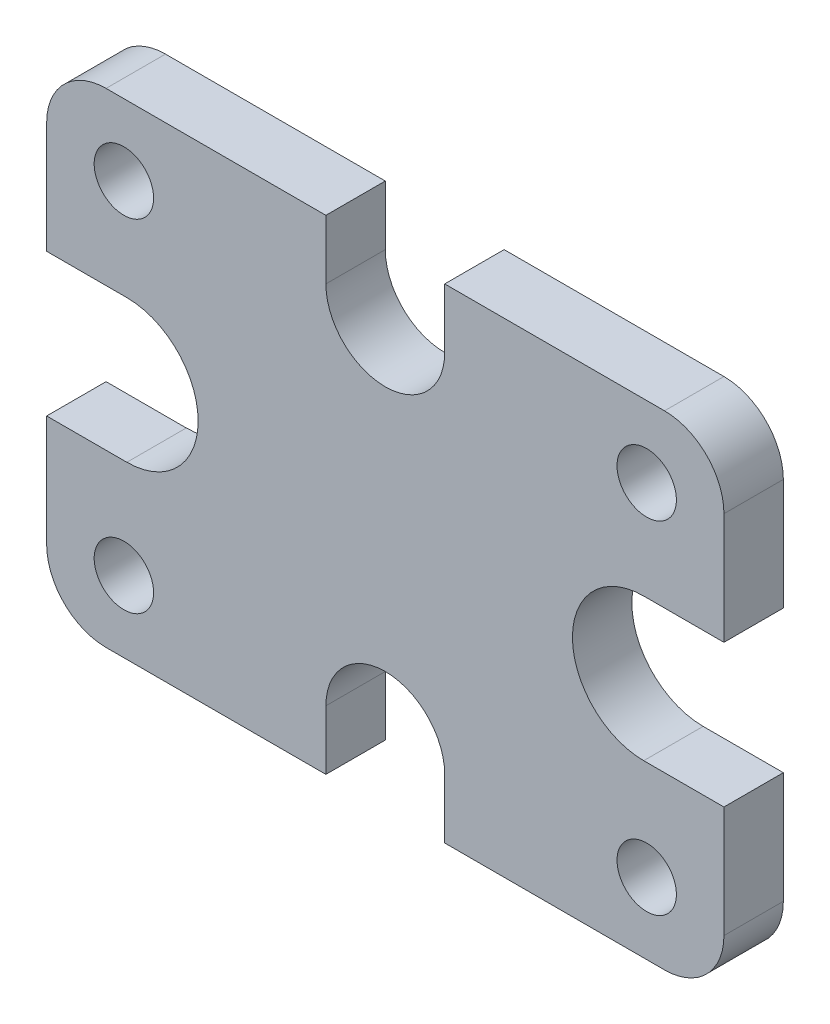
ISO-10303-21;
HEADER;
FILE_DESCRIPTION(('STEP AP214'),'2;1');
FILE_NAME('part.step','',(''),(''),'','','');
FILE_SCHEMA(('AUTOMOTIVE_DESIGN { 1 0 10303 214 1 1 1 1 }'));
ENDSEC;
DATA;
#1=APPLICATION_CONTEXT('core data for automotive mechanical design processes');
#2=APPLICATION_PROTOCOL_DEFINITION('international standard','automotive_design',2000,#1);
#3=PRODUCT_CONTEXT('',#1,'mechanical');
#4=PRODUCT('Part','Part','',(#3));
#5=PRODUCT_RELATED_PRODUCT_CATEGORY('part','',(#4));
#6=PRODUCT_DEFINITION_FORMATION('','',#4);
#7=PRODUCT_DEFINITION_CONTEXT('part definition',#1,'design');
#8=PRODUCT_DEFINITION('design','',#6,#7);
#9=PRODUCT_DEFINITION_SHAPE('','',#8);
#10=(LENGTH_UNIT() NAMED_UNIT(*) SI_UNIT(.MILLI.,.METRE.));
#11=(NAMED_UNIT(*) PLANE_ANGLE_UNIT() SI_UNIT($,.RADIAN.));
#12=(NAMED_UNIT(*) SI_UNIT($,.STERADIAN.) SOLID_ANGLE_UNIT());
#13=UNCERTAINTY_MEASURE_WITH_UNIT(LENGTH_MEASURE(1.E-05),#10,'distance_accuracy_value','');
#14=(GEOMETRIC_REPRESENTATION_CONTEXT(3) GLOBAL_UNCERTAINTY_ASSIGNED_CONTEXT((#13)) GLOBAL_UNIT_ASSIGNED_CONTEXT((#10,
#11,#12)) REPRESENTATION_CONTEXT('',''));
#15=CARTESIAN_POINT('',(0.,0.,0.));
#16=DIRECTION('',(0.,0.,1.));
#17=DIRECTION('',(1.,0.,0.));
#18=AXIS2_PLACEMENT_3D('',#15,#16,#17);
#19=CARTESIAN_POINT('',(10.0000000000001,0.,10.));
#20=DIRECTION('',(0.,1.,0.));
#21=DIRECTION('',(0.,0.,1.));
#22=AXIS2_PLACEMENT_3D('',#19,#20,#21);
#23=PLANE('',#22);
#24=DIRECTION('',(1.,0.,0.));
#25=VECTOR('',#24,1.);
#26=CARTESIAN_POINT('',(0.,0.,10.));
#27=LINE('',#26,#25);
#28=CARTESIAN_POINT('',(10.0000000000001,0.,10.));
#29=VERTEX_POINT('',#28);
#30=CARTESIAN_POINT('',(47.0000000000001,0.,10.));
#31=VERTEX_POINT('',#30);
#32=EDGE_CURVE('E199',#29,#31,#27,.T.);
#33=ORIENTED_EDGE('',*,*,#32,.F.);
#34=DIRECTION('',(0.,0.,-1.));
#35=VECTOR('',#34,1.);
#36=CARTESIAN_POINT('',(10.0000000000001,0.,10.));
#37=LINE('',#36,#35);
#38=CARTESIAN_POINT('',(10.0000000000001,0.,0.));
#39=VERTEX_POINT('',#38);
#40=EDGE_CURVE('E378',#29,#39,#37,.T.);
#41=ORIENTED_EDGE('',*,*,#40,.T.);
#42=DIRECTION('',(1.,0.,0.));
#43=VECTOR('',#42,1.);
#44=CARTESIAN_POINT('',(10.0000000000001,0.,0.));
#45=LINE('',#44,#43);
#46=CARTESIAN_POINT('',(47.0000000000001,0.,0.));
#47=VERTEX_POINT('',#46);
#48=EDGE_CURVE('E220',#39,#47,#45,.T.);
#49=ORIENTED_EDGE('',*,*,#48,.T.);
#50=DIRECTION('',(0.,0.,-1.));
#51=VECTOR('',#50,1.);
#52=CARTESIAN_POINT('',(47.0000000000001,0.,10.));
#53=LINE('',#52,#51);
#54=EDGE_CURVE('E214',#31,#47,#53,.T.);
#55=ORIENTED_EDGE('',*,*,#54,.F.);
#56=EDGE_LOOP('',(#33,#41,#49,#55));
#57=FACE_BOUND('',#56,.T.);
#58=ADVANCED_FACE('F39',(#57),#23,.F.);
#59=CARTESIAN_POINT('',(47.0000000000001,0.,10.));
#60=DIRECTION('',(-1.,0.,0.));
#61=DIRECTION('',(0.,0.,1.));
#62=AXIS2_PLACEMENT_3D('',#59,#60,#61);
#63=PLANE('',#62);
#64=DIRECTION('',(0.,1.,0.));
#65=VECTOR('',#64,1.);
#66=CARTESIAN_POINT('',(47.0000000000001,0.,0.));
#67=LINE('',#66,#65);
#68=CARTESIAN_POINT('',(47.0000000000001,10.,0.));
#69=VERTEX_POINT('',#68);
#70=EDGE_CURVE('E268',#47,#69,#67,.T.);
#71=ORIENTED_EDGE('',*,*,#70,.T.);
#72=DIRECTION('',(0.,0.,-1.));
#73=VECTOR('',#72,1.);
#74=CARTESIAN_POINT('',(47.0000000000001,10.,10.));
#75=LINE('',#74,#73);
#76=CARTESIAN_POINT('',(47.0000000000001,10.,10.));
#77=VERTEX_POINT('',#76);
#78=EDGE_CURVE('E222',#77,#69,#75,.T.);
#79=ORIENTED_EDGE('',*,*,#78,.F.);
#80=DIRECTION('',(0.,1.,0.));
#81=VECTOR('',#80,1.);
#82=CARTESIAN_POINT('',(47.0000000000001,0.,10.));
#83=LINE('',#82,#81);
#84=EDGE_CURVE('E202',#31,#77,#83,.T.);
#85=ORIENTED_EDGE('',*,*,#84,.F.);
#86=ORIENTED_EDGE('',*,*,#54,.T.);
#87=EDGE_LOOP('',(#71,#79,#85,#86));
#88=FACE_BOUND('',#87,.T.);
#89=ADVANCED_FACE('F224',(#88),#63,.F.);
#90=CARTESIAN_POINT('',(57.0000000000001,10.,10.));
#91=DIRECTION('',(0.,0.,-1.));
#92=DIRECTION('',(-1.,0.,0.));
#93=AXIS2_PLACEMENT_3D('',#90,#91,#92);
#94=CYLINDRICAL_SURFACE('',#93,10.);
#95=CARTESIAN_POINT('',(57.0000000000001,10.,0.));
#96=DIRECTION('',(0.,0.,-1.));
#97=DIRECTION('',(1.,0.,0.));
#98=AXIS2_PLACEMENT_3D('',#95,#96,#97);
#99=CIRCLE('',#98,10.);
#100=CARTESIAN_POINT('',(67.0000000000001,10.,0.));
#101=VERTEX_POINT('',#100);
#102=EDGE_CURVE('E271',#69,#101,#99,.T.);
#103=ORIENTED_EDGE('',*,*,#102,.T.);
#104=DIRECTION('',(0.,0.,-1.));
#105=VECTOR('',#104,1.);
#106=CARTESIAN_POINT('',(67.0000000000001,10.,10.));
#107=LINE('',#106,#105);
#108=CARTESIAN_POINT('',(67.0000000000001,10.,10.));
#109=VERTEX_POINT('',#108);
#110=EDGE_CURVE('E353',#109,#101,#107,.T.);
#111=ORIENTED_EDGE('',*,*,#110,.F.);
#112=CARTESIAN_POINT('',(57.0000000000001,10.,10.));
#113=DIRECTION('',(0.,0.,-1.));
#114=DIRECTION('',(1.,0.,0.));
#115=AXIS2_PLACEMENT_3D('',#112,#113,#114);
#116=CIRCLE('',#115,10.);
#117=EDGE_CURVE('E228',#77,#109,#116,.T.);
#118=ORIENTED_EDGE('',*,*,#117,.F.);
#119=ORIENTED_EDGE('',*,*,#78,.T.);
#120=EDGE_LOOP('',(#103,#111,#118,#119));
#121=FACE_BOUND('',#120,.T.);
#122=ADVANCED_FACE('F424',(#121),#94,.F.);
#123=CARTESIAN_POINT('',(67.0000000000001,10.,10.));
#124=DIRECTION('',(1.,0.,0.));
#125=DIRECTION('',(0.,0.,-1.));
#126=AXIS2_PLACEMENT_3D('',#123,#124,#125);
#127=PLANE('',#126);
#128=DIRECTION('',(0.,-1.,0.));
#129=VECTOR('',#128,1.);
#130=CARTESIAN_POINT('',(67.0000000000001,10.,0.));
#131=LINE('',#130,#129);
#132=CARTESIAN_POINT('',(67.0000000000001,0.,0.));
#133=VERTEX_POINT('',#132);
#134=EDGE_CURVE('E272',#101,#133,#131,.T.);
#135=ORIENTED_EDGE('',*,*,#134,.T.);
#136=DIRECTION('',(0.,0.,-1.));
#137=VECTOR('',#136,1.);
#138=CARTESIAN_POINT('',(67.0000000000001,0.,10.));
#139=LINE('',#138,#137);
#140=CARTESIAN_POINT('',(67.0000000000001,0.,10.));
#141=VERTEX_POINT('',#140);
#142=EDGE_CURVE('E346',#141,#133,#139,.T.);
#143=ORIENTED_EDGE('',*,*,#142,.F.);
#144=DIRECTION('',(0.,-1.,0.));
#145=VECTOR('',#144,1.);
#146=CARTESIAN_POINT('',(67.0000000000001,10.,10.));
#147=LINE('',#146,#145);
#148=EDGE_CURVE('E226',#109,#141,#147,.T.);
#149=ORIENTED_EDGE('',*,*,#148,.F.);
#150=ORIENTED_EDGE('',*,*,#110,.T.);
#151=EDGE_LOOP('',(#135,#143,#149,#150));
#152=FACE_BOUND('',#151,.T.);
#153=ADVANCED_FACE('F453',(#152),#127,.F.);
#154=CARTESIAN_POINT('',(114.,0.,10.));
#155=DIRECTION('',(0.,1.,0.));
#156=DIRECTION('',(0.,0.,1.));
#157=AXIS2_PLACEMENT_3D('',#154,#155,#156);
#158=PLANE('',#157);
#159=DIRECTION('',(1.,0.,0.));
#160=VECTOR('',#159,1.);
#161=CARTESIAN_POINT('',(114.,0.,0.));
#162=LINE('',#161,#160);
#163=CARTESIAN_POINT('',(104.,0.,0.));
#164=VERTEX_POINT('',#163);
#165=EDGE_CURVE('E277',#133,#164,#162,.T.);
#166=ORIENTED_EDGE('',*,*,#165,.T.);
#167=DIRECTION('',(0.,0.,-1.));
#168=VECTOR('',#167,1.);
#169=CARTESIAN_POINT('',(104.,0.,10.));
#170=LINE('',#169,#168);
#171=CARTESIAN_POINT('',(104.,0.,10.));
#172=VERTEX_POINT('',#171);
#173=EDGE_CURVE('E364',#164,#172,#170,.F.);
#174=ORIENTED_EDGE('',*,*,#173,.T.);
#175=DIRECTION('',(1.,0.,0.));
#176=VECTOR('',#175,1.);
#177=CARTESIAN_POINT('',(67.0000000000001,0.,10.));
#178=LINE('',#177,#176);
#179=EDGE_CURVE('E231',#141,#172,#178,.T.);
#180=ORIENTED_EDGE('',*,*,#179,.F.);
#181=ORIENTED_EDGE('',*,*,#142,.T.);
#182=EDGE_LOOP('',(#166,#174,#180,#181));
#183=FACE_BOUND('',#182,.T.);
#184=ADVANCED_FACE('F451',(#183),#158,.F.);
#185=CARTESIAN_POINT('',(114.,10.0000000000001,10.));
#186=DIRECTION('',(-1.,0.,0.));
#187=DIRECTION('',(0.,0.,1.));
#188=AXIS2_PLACEMENT_3D('',#185,#186,#187);
#189=PLANE('',#188);
#190=DIRECTION('',(0.,1.,0.));
#191=VECTOR('',#190,1.);
#192=CARTESIAN_POINT('',(114.,10.0000000000001,10.));
#193=LINE('',#192,#191);
#194=CARTESIAN_POINT('',(114.,10.0000000000001,10.));
#195=VERTEX_POINT('',#194);
#196=CARTESIAN_POINT('',(114.,28.7500000000001,10.));
#197=VERTEX_POINT('',#196);
#198=EDGE_CURVE('E232',#195,#197,#193,.T.);
#199=ORIENTED_EDGE('',*,*,#198,.F.);
#200=DIRECTION('',(0.,0.,-1.));
#201=VECTOR('',#200,1.);
#202=CARTESIAN_POINT('',(114.,10.0000000000001,10.));
#203=LINE('',#202,#201);
#204=CARTESIAN_POINT('',(114.,10.0000000000001,0.));
#205=VERTEX_POINT('',#204);
#206=EDGE_CURVE('E219',#195,#205,#203,.T.);
#207=ORIENTED_EDGE('',*,*,#206,.T.);
#208=DIRECTION('',(0.,1.,0.));
#209=VECTOR('',#208,1.);
#210=CARTESIAN_POINT('',(114.,10.0000000000001,0.));
#211=LINE('',#210,#209);
#212=CARTESIAN_POINT('',(114.,28.7500000000001,0.));
#213=VERTEX_POINT('',#212);
#214=EDGE_CURVE('E276',#205,#213,#211,.T.);
#215=ORIENTED_EDGE('',*,*,#214,.T.);
#216=DIRECTION('',(0.,0.,-1.));
#217=VECTOR('',#216,1.);
#218=CARTESIAN_POINT('',(114.,28.7500000000001,10.));
#219=LINE('',#218,#217);
#220=EDGE_CURVE('E342',#197,#213,#219,.T.);
#221=ORIENTED_EDGE('',*,*,#220,.F.);
#222=EDGE_LOOP('',(#199,#207,#215,#221));
#223=FACE_BOUND('',#222,.T.);
#224=ADVANCED_FACE('F459',(#223),#189,.F.);
#225=CARTESIAN_POINT('',(100.5,28.75,10.));
#226=DIRECTION('',(0.,-1.,0.));
#227=DIRECTION('',(1.,0.,0.));
#228=AXIS2_PLACEMENT_3D('',#225,#226,#227);
#229=PLANE('',#228);
#230=DIRECTION('',(-1.,0.,0.));
#231=VECTOR('',#230,1.);
#232=CARTESIAN_POINT('',(100.5,28.75,0.));
#233=LINE('',#232,#231);
#234=CARTESIAN_POINT('',(100.5,28.75,0.));
#235=VERTEX_POINT('',#234);
#236=EDGE_CURVE('E283',#213,#235,#233,.T.);
#237=ORIENTED_EDGE('',*,*,#236,.T.);
#238=DIRECTION('',(0.,0.,-1.));
#239=VECTOR('',#238,1.);
#240=CARTESIAN_POINT('',(100.5,28.75,10.));
#241=LINE('',#240,#239);
#242=CARTESIAN_POINT('',(100.5,28.75,10.));
#243=VERTEX_POINT('',#242);
#244=EDGE_CURVE('E345',#243,#235,#241,.T.);
#245=ORIENTED_EDGE('',*,*,#244,.F.);
#246=DIRECTION('',(-1.,0.,0.));
#247=VECTOR('',#246,1.);
#248=CARTESIAN_POINT('',(100.5,28.75,10.));
#249=LINE('',#248,#247);
#250=EDGE_CURVE('E240',#197,#243,#249,.T.);
#251=ORIENTED_EDGE('',*,*,#250,.F.);
#252=ORIENTED_EDGE('',*,*,#220,.T.);
#253=EDGE_LOOP('',(#237,#245,#251,#252));
#254=FACE_BOUND('',#253,.T.);
#255=ADVANCED_FACE('F464',(#254),#229,.F.);
#256=CARTESIAN_POINT('',(100.5,40.75,10.));
#257=DIRECTION('',(0.,0.,-1.));
#258=DIRECTION('',(-1.,0.,0.));
#259=AXIS2_PLACEMENT_3D('',#256,#257,#258);
#260=CYLINDRICAL_SURFACE('',#259,12.);
#261=CARTESIAN_POINT('',(100.5,40.75,0.));
#262=DIRECTION('',(0.,0.,-1.));
#263=DIRECTION('',(1.,0.,0.));
#264=AXIS2_PLACEMENT_3D('',#261,#262,#263);
#265=CIRCLE('',#264,12.);
#266=CARTESIAN_POINT('',(100.5,52.75,0.));
#267=VERTEX_POINT('',#266);
#268=EDGE_CURVE('E281',#235,#267,#265,.T.);
#269=ORIENTED_EDGE('',*,*,#268,.T.);
#270=DIRECTION('',(0.,0.,-1.));
#271=VECTOR('',#270,1.);
#272=CARTESIAN_POINT('',(100.5,52.75,10.));
#273=LINE('',#272,#271);
#274=CARTESIAN_POINT('',(100.5,52.75,10.));
#275=VERTEX_POINT('',#274);
#276=EDGE_CURVE('E339',#275,#267,#273,.T.);
#277=ORIENTED_EDGE('',*,*,#276,.F.);
#278=CARTESIAN_POINT('',(100.5,40.75,10.));
#279=DIRECTION('',(0.,0.,-1.));
#280=DIRECTION('',(1.,0.,0.));
#281=AXIS2_PLACEMENT_3D('',#278,#279,#280);
#282=CIRCLE('',#281,12.);
#283=EDGE_CURVE('E239',#243,#275,#282,.T.);
#284=ORIENTED_EDGE('',*,*,#283,.F.);
#285=ORIENTED_EDGE('',*,*,#244,.T.);
#286=EDGE_LOOP('',(#269,#277,#284,#285));
#287=FACE_BOUND('',#286,.T.);
#288=ADVANCED_FACE('F467',(#287),#260,.F.);
#289=CARTESIAN_POINT('',(100.5,52.75,10.));
#290=DIRECTION('',(0.,1.,0.));
#291=DIRECTION('',(-1.,0.,0.));
#292=AXIS2_PLACEMENT_3D('',#289,#290,#291);
#293=PLANE('',#292);
#294=DIRECTION('',(1.,0.,0.));
#295=VECTOR('',#294,1.);
#296=CARTESIAN_POINT('',(100.5,52.75,0.));
#297=LINE('',#296,#295);
#298=CARTESIAN_POINT('',(114.,52.7500000000001,0.));
#299=VERTEX_POINT('',#298);
#300=EDGE_CURVE('E282',#267,#299,#297,.T.);
#301=ORIENTED_EDGE('',*,*,#300,.T.);
#302=DIRECTION('',(0.,0.,-1.));
#303=VECTOR('',#302,1.);
#304=CARTESIAN_POINT('',(114.,52.7500000000001,10.));
#305=LINE('',#304,#303);
#306=CARTESIAN_POINT('',(114.,52.7500000000001,10.));
#307=VERTEX_POINT('',#306);
#308=EDGE_CURVE('E338',#307,#299,#305,.T.);
#309=ORIENTED_EDGE('',*,*,#308,.F.);
#310=DIRECTION('',(1.,0.,0.));
#311=VECTOR('',#310,1.);
#312=CARTESIAN_POINT('',(100.5,52.75,10.));
#313=LINE('',#312,#311);
#314=EDGE_CURVE('E243',#275,#307,#313,.T.);
#315=ORIENTED_EDGE('',*,*,#314,.F.);
#316=ORIENTED_EDGE('',*,*,#276,.T.);
#317=EDGE_LOOP('',(#301,#309,#315,#316));
#318=FACE_BOUND('',#317,.T.);
#319=ADVANCED_FACE('F475',(#318),#293,.F.);
#320=CARTESIAN_POINT('',(114.,81.5,10.));
#321=DIRECTION('',(-1.,0.,0.));
#322=DIRECTION('',(0.,0.,1.));
#323=AXIS2_PLACEMENT_3D('',#320,#321,#322);
#324=PLANE('',#323);
#325=DIRECTION('',(0.,1.,0.));
#326=VECTOR('',#325,1.);
#327=CARTESIAN_POINT('',(114.,81.5,0.));
#328=LINE('',#327,#326);
#329=CARTESIAN_POINT('',(114.,71.5,0.));
#330=VERTEX_POINT('',#329);
#331=EDGE_CURVE('E286',#299,#330,#328,.T.);
#332=ORIENTED_EDGE('',*,*,#331,.T.);
#333=DIRECTION('',(0.,0.,-1.));
#334=VECTOR('',#333,1.);
#335=CARTESIAN_POINT('',(114.,71.5,10.));
#336=LINE('',#335,#334);
#337=CARTESIAN_POINT('',(114.,71.5,10.));
#338=VERTEX_POINT('',#337);
#339=EDGE_CURVE('E376',#330,#338,#336,.F.);
#340=ORIENTED_EDGE('',*,*,#339,.T.);
#341=DIRECTION('',(0.,1.,0.));
#342=VECTOR('',#341,1.);
#343=CARTESIAN_POINT('',(114.,52.7500000000001,10.));
#344=LINE('',#343,#342);
#345=EDGE_CURVE('E241',#307,#338,#344,.T.);
#346=ORIENTED_EDGE('',*,*,#345,.F.);
#347=ORIENTED_EDGE('',*,*,#308,.T.);
#348=EDGE_LOOP('',(#332,#340,#346,#347));
#349=FACE_BOUND('',#348,.T.);
#350=ADVANCED_FACE('F480',(#349),#324,.F.);
#351=CARTESIAN_POINT('',(104.,81.5,10.));
#352=DIRECTION('',(0.,-1.,0.));
#353=DIRECTION('',(0.,0.,-1.));
#354=AXIS2_PLACEMENT_3D('',#351,#352,#353);
#355=PLANE('',#354);
#356=DIRECTION('',(-1.,0.,0.));
#357=VECTOR('',#356,1.);
#358=CARTESIAN_POINT('',(104.,81.5,10.));
#359=LINE('',#358,#357);
#360=CARTESIAN_POINT('',(104.,81.5,10.));
#361=VERTEX_POINT('',#360);
#362=CARTESIAN_POINT('',(67.0000000000001,81.5,10.));
#363=VERTEX_POINT('',#362);
#364=EDGE_CURVE('E248',#361,#363,#359,.T.);
#365=ORIENTED_EDGE('',*,*,#364,.F.);
#366=DIRECTION('',(0.,0.,-1.));
#367=VECTOR('',#366,1.);
#368=CARTESIAN_POINT('',(104.,81.5,10.));
#369=LINE('',#368,#367);
#370=CARTESIAN_POINT('',(104.,81.5,0.));
#371=VERTEX_POINT('',#370);
#372=EDGE_CURVE('E373',#361,#371,#369,.T.);
#373=ORIENTED_EDGE('',*,*,#372,.T.);
#374=DIRECTION('',(-1.,0.,0.));
#375=VECTOR('',#374,1.);
#376=CARTESIAN_POINT('',(104.,81.5,0.));
#377=LINE('',#376,#375);
#378=CARTESIAN_POINT('',(67.0000000000001,81.5,0.));
#379=VERTEX_POINT('',#378);
#380=EDGE_CURVE('E292',#371,#379,#377,.T.);
#381=ORIENTED_EDGE('',*,*,#380,.T.);
#382=DIRECTION('',(0.,0.,-1.));
#383=VECTOR('',#382,1.);
#384=CARTESIAN_POINT('',(67.0000000000001,81.5,10.));
#385=LINE('',#384,#383);
#386=EDGE_CURVE('E334',#363,#379,#385,.T.);
#387=ORIENTED_EDGE('',*,*,#386,.F.);
#388=EDGE_LOOP('',(#365,#373,#381,#387));
#389=FACE_BOUND('',#388,.T.);
#390=ADVANCED_FACE('F482',(#389),#355,.F.);
#391=CARTESIAN_POINT('',(67.0000000000001,81.5,10.));
#392=DIRECTION('',(1.,0.,0.));
#393=DIRECTION('',(0.,0.,-1.));
#394=AXIS2_PLACEMENT_3D('',#391,#392,#393);
#395=PLANE('',#394);
#396=DIRECTION('',(0.,-1.,0.));
#397=VECTOR('',#396,1.);
#398=CARTESIAN_POINT('',(67.0000000000001,81.5,0.));
#399=LINE('',#398,#397);
#400=CARTESIAN_POINT('',(67.0000000000001,71.5,0.));
#401=VERTEX_POINT('',#400);
#402=EDGE_CURVE('E291',#379,#401,#399,.T.);
#403=ORIENTED_EDGE('',*,*,#402,.T.);
#404=DIRECTION('',(0.,0.,-1.));
#405=VECTOR('',#404,1.);
#406=CARTESIAN_POINT('',(67.0000000000001,71.5,10.));
#407=LINE('',#406,#405);
#408=CARTESIAN_POINT('',(67.0000000000001,71.5,10.));
#409=VERTEX_POINT('',#408);
#410=EDGE_CURVE('E329',#409,#401,#407,.T.);
#411=ORIENTED_EDGE('',*,*,#410,.F.);
#412=DIRECTION('',(0.,-1.,0.));
#413=VECTOR('',#412,1.);
#414=CARTESIAN_POINT('',(67.0000000000001,81.5,10.));
#415=LINE('',#414,#413);
#416=EDGE_CURVE('E246',#363,#409,#415,.T.);
#417=ORIENTED_EDGE('',*,*,#416,.F.);
#418=ORIENTED_EDGE('',*,*,#386,.T.);
#419=EDGE_LOOP('',(#403,#411,#417,#418));
#420=FACE_BOUND('',#419,.T.);
#421=ADVANCED_FACE('F491',(#420),#395,.F.);
#422=CARTESIAN_POINT('',(57.0000000000001,71.5,10.));
#423=DIRECTION('',(0.,0.,-1.));
#424=DIRECTION('',(-1.,0.,0.));
#425=AXIS2_PLACEMENT_3D('',#422,#423,#424);
#426=CYLINDRICAL_SURFACE('',#425,10.);
#427=CARTESIAN_POINT('',(57.0000000000001,71.5,0.));
#428=DIRECTION('',(0.,0.,-1.));
#429=DIRECTION('',(1.,0.,0.));
#430=AXIS2_PLACEMENT_3D('',#427,#428,#429);
#431=CIRCLE('',#430,10.);
#432=CARTESIAN_POINT('',(47.0000000000001,71.5,0.));
#433=VERTEX_POINT('',#432);
#434=EDGE_CURVE('E293',#401,#433,#431,.T.);
#435=ORIENTED_EDGE('',*,*,#434,.T.);
#436=DIRECTION('',(0.,0.,-1.));
#437=VECTOR('',#436,1.);
#438=CARTESIAN_POINT('',(47.0000000000001,71.5,10.));
#439=LINE('',#438,#437);
#440=CARTESIAN_POINT('',(47.0000000000001,71.5,10.));
#441=VERTEX_POINT('',#440);
#442=EDGE_CURVE('E330',#441,#433,#439,.T.);
#443=ORIENTED_EDGE('',*,*,#442,.F.);
#444=CARTESIAN_POINT('',(57.0000000000001,71.5,10.));
#445=DIRECTION('',(0.,0.,-1.));
#446=DIRECTION('',(1.,0.,0.));
#447=AXIS2_PLACEMENT_3D('',#444,#445,#446);
#448=CIRCLE('',#447,10.);
#449=EDGE_CURVE('E247',#409,#441,#448,.T.);
#450=ORIENTED_EDGE('',*,*,#449,.F.);
#451=ORIENTED_EDGE('',*,*,#410,.T.);
#452=EDGE_LOOP('',(#435,#443,#450,#451));
#453=FACE_BOUND('',#452,.T.);
#454=ADVANCED_FACE('F494',(#453),#426,.F.);
#455=CARTESIAN_POINT('',(47.0000000000001,71.5,10.));
#456=DIRECTION('',(-1.,0.,0.));
#457=DIRECTION('',(0.,0.,1.));
#458=AXIS2_PLACEMENT_3D('',#455,#456,#457);
#459=PLANE('',#458);
#460=DIRECTION('',(0.,1.,0.));
#461=VECTOR('',#460,1.);
#462=CARTESIAN_POINT('',(47.0000000000001,71.5,0.));
#463=LINE('',#462,#461);
#464=CARTESIAN_POINT('',(47.0000000000001,81.5,0.));
#465=VERTEX_POINT('',#464);
#466=EDGE_CURVE('E300',#433,#465,#463,.T.);
#467=ORIENTED_EDGE('',*,*,#466,.T.);
#468=DIRECTION('',(0.,0.,-1.));
#469=VECTOR('',#468,1.);
#470=CARTESIAN_POINT('',(47.0000000000001,81.5,10.));
#471=LINE('',#470,#469);
#472=CARTESIAN_POINT('',(47.0000000000001,81.5,10.));
#473=VERTEX_POINT('',#472);
#474=EDGE_CURVE('E322',#473,#465,#471,.T.);
#475=ORIENTED_EDGE('',*,*,#474,.F.);
#476=DIRECTION('',(0.,1.,0.));
#477=VECTOR('',#476,1.);
#478=CARTESIAN_POINT('',(47.0000000000001,71.5,10.));
#479=LINE('',#478,#477);
#480=EDGE_CURVE('E252',#441,#473,#479,.T.);
#481=ORIENTED_EDGE('',*,*,#480,.F.);
#482=ORIENTED_EDGE('',*,*,#442,.T.);
#483=EDGE_LOOP('',(#467,#475,#481,#482));
#484=FACE_BOUND('',#483,.T.);
#485=ADVANCED_FACE('F503',(#484),#459,.F.);
#486=CARTESIAN_POINT('',(0.,81.5,10.));
#487=DIRECTION('',(0.,-1.,0.));
#488=DIRECTION('',(0.,0.,-1.));
#489=AXIS2_PLACEMENT_3D('',#486,#487,#488);
#490=PLANE('',#489);
#491=DIRECTION('',(-1.,0.,0.));
#492=VECTOR('',#491,1.);
#493=CARTESIAN_POINT('',(0.,81.5,0.));
#494=LINE('',#493,#492);
#495=CARTESIAN_POINT('',(10.,81.5,0.));
#496=VERTEX_POINT('',#495);
#497=EDGE_CURVE('E297',#465,#496,#494,.T.);
#498=ORIENTED_EDGE('',*,*,#497,.T.);
#499=DIRECTION('',(0.,0.,-1.));
#500=VECTOR('',#499,1.);
#501=CARTESIAN_POINT('',(10.,81.5,10.));
#502=LINE('',#501,#500);
#503=CARTESIAN_POINT('',(10.,81.5,10.));
#504=VERTEX_POINT('',#503);
#505=EDGE_CURVE('E11',#496,#504,#502,.F.);
#506=ORIENTED_EDGE('',*,*,#505,.T.);
#507=DIRECTION('',(-1.,0.,0.));
#508=VECTOR('',#507,1.);
#509=CARTESIAN_POINT('',(47.0000000000001,81.5,10.));
#510=LINE('',#509,#508);
#511=EDGE_CURVE('E255',#473,#504,#510,.T.);
#512=ORIENTED_EDGE('',*,*,#511,.F.);
#513=ORIENTED_EDGE('',*,*,#474,.T.);
#514=EDGE_LOOP('',(#498,#506,#512,#513));
#515=FACE_BOUND('',#514,.T.);
#516=ADVANCED_FACE('F501',(#515),#490,.F.);
#517=CARTESIAN_POINT('',(0.,71.4999999999999,10.));
#518=DIRECTION('',(1.,0.,0.));
#519=DIRECTION('',(0.,0.,-1.));
#520=AXIS2_PLACEMENT_3D('',#517,#518,#519);
#521=PLANE('',#520);
#522=DIRECTION('',(0.,-1.,0.));
#523=VECTOR('',#522,1.);
#524=CARTESIAN_POINT('',(0.,71.4999999999999,10.));
#525=LINE('',#524,#523);
#526=CARTESIAN_POINT('',(0.,71.4999999999999,10.));
#527=VERTEX_POINT('',#526);
#528=CARTESIAN_POINT('',(0.,52.75,10.));
#529=VERTEX_POINT('',#528);
#530=EDGE_CURVE('E258',#527,#529,#525,.T.);
#531=ORIENTED_EDGE('',*,*,#530,.F.);
#532=DIRECTION('',(0.,0.,-1.));
#533=VECTOR('',#532,1.);
#534=CARTESIAN_POINT('',(0.,71.4999999999999,10.));
#535=LINE('',#534,#533);
#536=CARTESIAN_POINT('',(0.,71.4999999999999,0.));
#537=VERTEX_POINT('',#536);
#538=EDGE_CURVE('E50',#527,#537,#535,.T.);
#539=ORIENTED_EDGE('',*,*,#538,.T.);
#540=DIRECTION('',(0.,-1.,0.));
#541=VECTOR('',#540,1.);
#542=CARTESIAN_POINT('',(0.,71.4999999999999,0.));
#543=LINE('',#542,#541);
#544=CARTESIAN_POINT('',(0.,52.75,0.));
#545=VERTEX_POINT('',#544);
#546=EDGE_CURVE('E301',#537,#545,#543,.T.);
#547=ORIENTED_EDGE('',*,*,#546,.T.);
#548=DIRECTION('',(0.,0.,-1.));
#549=VECTOR('',#548,1.);
#550=CARTESIAN_POINT('',(0.,52.75,10.));
#551=LINE('',#550,#549);
#552=EDGE_CURVE('E321',#529,#545,#551,.T.);
#553=ORIENTED_EDGE('',*,*,#552,.F.);
#554=EDGE_LOOP('',(#531,#539,#547,#553));
#555=FACE_BOUND('',#554,.T.);
#556=ADVANCED_FACE('F383',(#555),#521,.F.);
#557=CARTESIAN_POINT('',(0.,52.75,10.));
#558=DIRECTION('',(0.,1.,0.));
#559=DIRECTION('',(0.,0.,1.));
#560=AXIS2_PLACEMENT_3D('',#557,#558,#559);
#561=PLANE('',#560);
#562=DIRECTION('',(1.,0.,0.));
#563=VECTOR('',#562,1.);
#564=CARTESIAN_POINT('',(0.,52.75,0.));
#565=LINE('',#564,#563);
#566=CARTESIAN_POINT('',(13.5,52.75,0.));
#567=VERTEX_POINT('',#566);
#568=EDGE_CURVE('E302',#545,#567,#565,.T.);
#569=ORIENTED_EDGE('',*,*,#568,.T.);
#570=DIRECTION('',(0.,0.,-1.));
#571=VECTOR('',#570,1.);
#572=CARTESIAN_POINT('',(13.5,52.75,10.));
#573=LINE('',#572,#571);
#574=CARTESIAN_POINT('',(13.5,52.75,10.));
#575=VERTEX_POINT('',#574);
#576=EDGE_CURVE('E318',#575,#567,#573,.T.);
#577=ORIENTED_EDGE('',*,*,#576,.F.);
#578=DIRECTION('',(1.,0.,0.));
#579=VECTOR('',#578,1.);
#580=CARTESIAN_POINT('',(0.,52.75,10.));
#581=LINE('',#580,#579);
#582=EDGE_CURVE('E256',#529,#575,#581,.T.);
#583=ORIENTED_EDGE('',*,*,#582,.F.);
#584=ORIENTED_EDGE('',*,*,#552,.T.);
#585=EDGE_LOOP('',(#569,#577,#583,#584));
#586=FACE_BOUND('',#585,.T.);
#587=ADVANCED_FACE('F392',(#586),#561,.F.);
#588=CARTESIAN_POINT('',(13.5,40.75,10.));
#589=DIRECTION('',(0.,0.,-1.));
#590=DIRECTION('',(-1.,0.,0.));
#591=AXIS2_PLACEMENT_3D('',#588,#589,#590);
#592=CYLINDRICAL_SURFACE('',#591,12.);
#593=CARTESIAN_POINT('',(13.5,40.75,0.));
#594=DIRECTION('',(0.,0.,-1.));
#595=DIRECTION('',(1.,0.,0.));
#596=AXIS2_PLACEMENT_3D('',#593,#594,#595);
#597=CIRCLE('',#596,12.);
#598=CARTESIAN_POINT('',(13.5,28.75,0.));
#599=VERTEX_POINT('',#598);
#600=EDGE_CURVE('E307',#567,#599,#597,.T.);
#601=ORIENTED_EDGE('',*,*,#600,.T.);
#602=DIRECTION('',(0.,0.,-1.));
#603=VECTOR('',#602,1.);
#604=CARTESIAN_POINT('',(13.5,28.75,10.));
#605=LINE('',#604,#603);
#606=CARTESIAN_POINT('',(13.5,28.75,10.));
#607=VERTEX_POINT('',#606);
#608=EDGE_CURVE('E312',#607,#599,#605,.T.);
#609=ORIENTED_EDGE('',*,*,#608,.F.);
#610=CARTESIAN_POINT('',(13.5,40.75,10.));
#611=DIRECTION('',(0.,0.,-1.));
#612=DIRECTION('',(1.,0.,0.));
#613=AXIS2_PLACEMENT_3D('',#610,#611,#612);
#614=CIRCLE('',#613,12.);
#615=EDGE_CURVE('E257',#575,#607,#614,.T.);
#616=ORIENTED_EDGE('',*,*,#615,.F.);
#617=ORIENTED_EDGE('',*,*,#576,.T.);
#618=EDGE_LOOP('',(#601,#609,#616,#617));
#619=FACE_BOUND('',#618,.T.);
#620=ADVANCED_FACE('F399',(#619),#592,.F.);
#621=CARTESIAN_POINT('',(13.5,28.75,10.));
#622=DIRECTION('',(0.,-1.,0.));
#623=DIRECTION('',(0.,0.,-1.));
#624=AXIS2_PLACEMENT_3D('',#621,#622,#623);
#625=PLANE('',#624);
#626=DIRECTION('',(-1.,0.,0.));
#627=VECTOR('',#626,1.);
#628=CARTESIAN_POINT('',(13.5,28.75,0.));
#629=LINE('',#628,#627);
#630=CARTESIAN_POINT('',(0.,28.75,0.));
#631=VERTEX_POINT('',#630);
#632=EDGE_CURVE('E310',#599,#631,#629,.T.);
#633=ORIENTED_EDGE('',*,*,#632,.T.);
#634=DIRECTION('',(0.,0.,-1.));
#635=VECTOR('',#634,1.);
#636=CARTESIAN_POINT('',(0.,28.75,10.));
#637=LINE('',#636,#635);
#638=CARTESIAN_POINT('',(0.,28.75,10.));
#639=VERTEX_POINT('',#638);
#640=EDGE_CURVE('E266',#639,#631,#637,.T.);
#641=ORIENTED_EDGE('',*,*,#640,.F.);
#642=DIRECTION('',(-1.,0.,0.));
#643=VECTOR('',#642,1.);
#644=CARTESIAN_POINT('',(13.5,28.75,10.));
#645=LINE('',#644,#643);
#646=EDGE_CURVE('E265',#607,#639,#645,.T.);
#647=ORIENTED_EDGE('',*,*,#646,.F.);
#648=ORIENTED_EDGE('',*,*,#608,.T.);
#649=EDGE_LOOP('',(#633,#641,#647,#648));
#650=FACE_BOUND('',#649,.T.);
#651=ADVANCED_FACE('F404',(#650),#625,.F.);
#652=CARTESIAN_POINT('',(0.,10.0000000000001,10.));
#653=DIRECTION('',(1.,0.,0.));
#654=DIRECTION('',(0.,0.,-1.));
#655=AXIS2_PLACEMENT_3D('',#652,#653,#654);
#656=PLANE('',#655);
#657=DIRECTION('',(0.,-1.,0.));
#658=VECTOR('',#657,1.);
#659=CARTESIAN_POINT('',(0.,10.0000000000001,0.));
#660=LINE('',#659,#658);
#661=CARTESIAN_POINT('',(0.,10.,0.));
#662=VERTEX_POINT('',#661);
#663=EDGE_CURVE('E215',#631,#662,#660,.T.);
#664=ORIENTED_EDGE('',*,*,#663,.T.);
#665=DIRECTION('',(0.,0.,-1.));
#666=VECTOR('',#665,1.);
#667=CARTESIAN_POINT('',(0.,10.0000000000001,10.));
#668=LINE('',#667,#666);
#669=CARTESIAN_POINT('',(0.,10.,10.));
#670=VERTEX_POINT('',#669);
#671=EDGE_CURVE('E53',#662,#670,#668,.F.);
#672=ORIENTED_EDGE('',*,*,#671,.T.);
#673=DIRECTION('',(0.,-1.,0.));
#674=VECTOR('',#673,1.);
#675=CARTESIAN_POINT('',(0.,28.75,10.));
#676=LINE('',#675,#674);
#677=EDGE_CURVE('E262',#639,#670,#676,.T.);
#678=ORIENTED_EDGE('',*,*,#677,.F.);
#679=ORIENTED_EDGE('',*,*,#640,.T.);
#680=EDGE_LOOP('',(#664,#672,#678,#679));
#681=FACE_BOUND('',#680,.T.);
#682=ADVANCED_FACE('F403',(#681),#656,.F.);
#683=CARTESIAN_POINT('',(57.0000000000001,10.,10.));
#684=DIRECTION('',(0.,0.,1.));
#685=DIRECTION('',(1.,0.,0.));
#686=AXIS2_PLACEMENT_3D('',#683,#684,#685);
#687=PLANE('',#686);
#688=CARTESIAN_POINT('',(13.,12.,10.));
#689=DIRECTION('',(0.,0.,1.));
#690=DIRECTION('',(1.,0.,0.));
#691=AXIS2_PLACEMENT_3D('',#688,#689,#690);
#692=CIRCLE('',#691,5.);
#693=CARTESIAN_POINT('',(18.,12.,10.));
#694=VERTEX_POINT('',#693);
#695=EDGE_CURVE('E766',#694,#694,#692,.T.);
#696=ORIENTED_EDGE('',*,*,#695,.F.);
#697=EDGE_LOOP('',(#696));
#698=FACE_BOUND('',#697,.T.);
#699=CARTESIAN_POINT('',(101.,12.,10.));
#700=DIRECTION('',(0.,0.,1.));
#701=DIRECTION('',(1.,0.,0.));
#702=AXIS2_PLACEMENT_3D('',#699,#700,#701);
#703=CIRCLE('',#702,5.);
#704=CARTESIAN_POINT('',(106.,12.,10.));
#705=VERTEX_POINT('',#704);
#706=EDGE_CURVE('E769',#705,#705,#703,.T.);
#707=ORIENTED_EDGE('',*,*,#706,.F.);
#708=EDGE_LOOP('',(#707));
#709=FACE_BOUND('',#708,.T.);
#710=CARTESIAN_POINT('',(101.,69.5,10.));
#711=DIRECTION('',(0.,0.,1.));
#712=DIRECTION('',(1.,0.,0.));
#713=AXIS2_PLACEMENT_3D('',#710,#711,#712);
#714=CIRCLE('',#713,5.00000000000001);
#715=CARTESIAN_POINT('',(106.,69.5,10.));
#716=VERTEX_POINT('',#715);
#717=EDGE_CURVE('E771',#716,#716,#714,.T.);
#718=ORIENTED_EDGE('',*,*,#717,.F.);
#719=EDGE_LOOP('',(#718));
#720=FACE_BOUND('',#719,.T.);
#721=CARTESIAN_POINT('',(13.,69.5,10.));
#722=DIRECTION('',(0.,0.,1.));
#723=DIRECTION('',(1.,0.,0.));
#724=AXIS2_PLACEMENT_3D('',#721,#722,#723);
#725=CIRCLE('',#724,5.00000000000001);
#726=CARTESIAN_POINT('',(18.,69.5,10.));
#727=VERTEX_POINT('',#726);
#728=EDGE_CURVE('E765',#727,#727,#725,.T.);
#729=ORIENTED_EDGE('',*,*,#728,.F.);
#730=EDGE_LOOP('',(#729));
#731=FACE_BOUND('',#730,.T.);
#732=ORIENTED_EDGE('',*,*,#179,.T.);
#733=CARTESIAN_POINT('',(104.,10.0000000000001,10.));
#734=DIRECTION('',(0.,0.,1.));
#735=DIRECTION('',(1.,0.,0.));
#736=AXIS2_PLACEMENT_3D('',#733,#734,#735);
#737=CIRCLE('',#736,10.);
#738=EDGE_CURVE('E371',#172,#195,#737,.T.);
#739=ORIENTED_EDGE('',*,*,#738,.T.);
#740=ORIENTED_EDGE('',*,*,#198,.T.);
#741=ORIENTED_EDGE('',*,*,#250,.T.);
#742=ORIENTED_EDGE('',*,*,#283,.T.);
#743=ORIENTED_EDGE('',*,*,#314,.T.);
#744=ORIENTED_EDGE('',*,*,#345,.T.);
#745=CARTESIAN_POINT('',(104.,71.5,10.));
#746=DIRECTION('',(0.,0.,1.));
#747=DIRECTION('',(1.,0.,0.));
#748=AXIS2_PLACEMENT_3D('',#745,#746,#747);
#749=CIRCLE('',#748,10.);
#750=EDGE_CURVE('E369',#338,#361,#749,.T.);
#751=ORIENTED_EDGE('',*,*,#750,.T.);
#752=ORIENTED_EDGE('',*,*,#364,.T.);
#753=ORIENTED_EDGE('',*,*,#416,.T.);
#754=ORIENTED_EDGE('',*,*,#449,.T.);
#755=ORIENTED_EDGE('',*,*,#480,.T.);
#756=ORIENTED_EDGE('',*,*,#511,.T.);
#757=CARTESIAN_POINT('',(10.,71.4999999999999,10.));
#758=DIRECTION('',(0.,0.,1.));
#759=DIRECTION('',(1.,0.,0.));
#760=AXIS2_PLACEMENT_3D('',#757,#758,#759);
#761=CIRCLE('',#760,10.);
#762=EDGE_CURVE('E65',#504,#527,#761,.T.);
#763=ORIENTED_EDGE('',*,*,#762,.T.);
#764=ORIENTED_EDGE('',*,*,#530,.T.);
#765=ORIENTED_EDGE('',*,*,#582,.T.);
#766=ORIENTED_EDGE('',*,*,#615,.T.);
#767=ORIENTED_EDGE('',*,*,#646,.T.);
#768=ORIENTED_EDGE('',*,*,#677,.T.);
#769=CARTESIAN_POINT('',(10.0000000000001,10.,10.));
#770=DIRECTION('',(0.,0.,1.));
#771=DIRECTION('',(1.,0.,0.));
#772=AXIS2_PLACEMENT_3D('',#769,#770,#771);
#773=CIRCLE('',#772,10.);
#774=EDGE_CURVE('E208',#670,#29,#773,.T.);
#775=ORIENTED_EDGE('',*,*,#774,.T.);
#776=ORIENTED_EDGE('',*,*,#32,.T.);
#777=ORIENTED_EDGE('',*,*,#84,.T.);
#778=ORIENTED_EDGE('',*,*,#117,.T.);
#779=ORIENTED_EDGE('',*,*,#148,.T.);
#780=EDGE_LOOP('',(#732,#739,#740,#741,#742,#743,#744,#751,#752,#753,#754,#755,#756,#763,#764,
#765,#766,#767,#768,#775,#776,#777,#778,#779));
#781=FACE_BOUND('',#780,.T.);
#782=ADVANCED_FACE('F201',(#698,#709,#720,#731,#781),#687,.T.);
#783=CARTESIAN_POINT('',(57.0000000000001,10.,0.));
#784=DIRECTION('',(0.,0.,1.));
#785=DIRECTION('',(1.,0.,0.));
#786=AXIS2_PLACEMENT_3D('',#783,#784,#785);
#787=PLANE('',#786);
#788=CARTESIAN_POINT('',(13.,12.,0.));
#789=DIRECTION('',(0.,0.,1.));
#790=DIRECTION('',(1.,0.,0.));
#791=AXIS2_PLACEMENT_3D('',#788,#789,#790);
#792=CIRCLE('',#791,5.);
#793=CARTESIAN_POINT('',(18.,12.,0.));
#794=VERTEX_POINT('',#793);
#795=EDGE_CURVE('E753',#794,#794,#792,.T.);
#796=ORIENTED_EDGE('',*,*,#795,.T.);
#797=EDGE_LOOP('',(#796));
#798=FACE_BOUND('',#797,.T.);
#799=CARTESIAN_POINT('',(101.,12.,0.));
#800=DIRECTION('',(0.,0.,1.));
#801=DIRECTION('',(1.,0.,0.));
#802=AXIS2_PLACEMENT_3D('',#799,#800,#801);
#803=CIRCLE('',#802,5.);
#804=CARTESIAN_POINT('',(106.,12.,0.));
#805=VERTEX_POINT('',#804);
#806=EDGE_CURVE('E752',#805,#805,#803,.T.);
#807=ORIENTED_EDGE('',*,*,#806,.T.);
#808=EDGE_LOOP('',(#807));
#809=FACE_BOUND('',#808,.T.);
#810=CARTESIAN_POINT('',(101.,69.5,0.));
#811=DIRECTION('',(0.,0.,1.));
#812=DIRECTION('',(1.,0.,0.));
#813=AXIS2_PLACEMENT_3D('',#810,#811,#812);
#814=CIRCLE('',#813,5.00000000000001);
#815=CARTESIAN_POINT('',(106.,69.5,0.));
#816=VERTEX_POINT('',#815);
#817=EDGE_CURVE('E757',#816,#816,#814,.T.);
#818=ORIENTED_EDGE('',*,*,#817,.T.);
#819=EDGE_LOOP('',(#818));
#820=FACE_BOUND('',#819,.T.);
#821=CARTESIAN_POINT('',(13.,69.5,0.));
#822=DIRECTION('',(0.,0.,1.));
#823=DIRECTION('',(1.,0.,0.));
#824=AXIS2_PLACEMENT_3D('',#821,#822,#823);
#825=CIRCLE('',#824,5.00000000000001);
#826=CARTESIAN_POINT('',(18.,69.5,0.));
#827=VERTEX_POINT('',#826);
#828=EDGE_CURVE('E267',#827,#827,#825,.T.);
#829=ORIENTED_EDGE('',*,*,#828,.T.);
#830=EDGE_LOOP('',(#829));
#831=FACE_BOUND('',#830,.T.);
#832=ORIENTED_EDGE('',*,*,#214,.F.);
#833=CARTESIAN_POINT('',(104.,10.0000000000001,0.));
#834=DIRECTION('',(0.,0.,1.));
#835=DIRECTION('',(1.,0.,0.));
#836=AXIS2_PLACEMENT_3D('',#833,#834,#835);
#837=CIRCLE('',#836,10.);
#838=EDGE_CURVE('E361',#205,#164,#837,.F.);
#839=ORIENTED_EDGE('',*,*,#838,.T.);
#840=ORIENTED_EDGE('',*,*,#165,.F.);
#841=ORIENTED_EDGE('',*,*,#134,.F.);
#842=ORIENTED_EDGE('',*,*,#102,.F.);
#843=ORIENTED_EDGE('',*,*,#70,.F.);
#844=ORIENTED_EDGE('',*,*,#48,.F.);
#845=CARTESIAN_POINT('',(10.0000000000001,10.,0.));
#846=DIRECTION('',(0.,0.,1.));
#847=DIRECTION('',(1.,0.,0.));
#848=AXIS2_PLACEMENT_3D('',#845,#846,#847);
#849=CIRCLE('',#848,10.);
#850=EDGE_CURVE('E359',#39,#662,#849,.F.);
#851=ORIENTED_EDGE('',*,*,#850,.T.);
#852=ORIENTED_EDGE('',*,*,#663,.F.);
#853=ORIENTED_EDGE('',*,*,#632,.F.);
#854=ORIENTED_EDGE('',*,*,#600,.F.);
#855=ORIENTED_EDGE('',*,*,#568,.F.);
#856=ORIENTED_EDGE('',*,*,#546,.F.);
#857=CARTESIAN_POINT('',(10.,71.4999999999999,0.));
#858=DIRECTION('',(0.,0.,1.));
#859=DIRECTION('',(1.,0.,0.));
#860=AXIS2_PLACEMENT_3D('',#857,#858,#859);
#861=CIRCLE('',#860,10.);
#862=EDGE_CURVE('E360',#537,#496,#861,.F.);
#863=ORIENTED_EDGE('',*,*,#862,.T.);
#864=ORIENTED_EDGE('',*,*,#497,.F.);
#865=ORIENTED_EDGE('',*,*,#466,.F.);
#866=ORIENTED_EDGE('',*,*,#434,.F.);
#867=ORIENTED_EDGE('',*,*,#402,.F.);
#868=ORIENTED_EDGE('',*,*,#380,.F.);
#869=CARTESIAN_POINT('',(104.,71.5,0.));
#870=DIRECTION('',(0.,0.,1.));
#871=DIRECTION('',(1.,0.,0.));
#872=AXIS2_PLACEMENT_3D('',#869,#870,#871);
#873=CIRCLE('',#872,10.);
#874=EDGE_CURVE('E363',#371,#330,#873,.F.);
#875=ORIENTED_EDGE('',*,*,#874,.T.);
#876=ORIENTED_EDGE('',*,*,#331,.F.);
#877=ORIENTED_EDGE('',*,*,#300,.F.);
#878=ORIENTED_EDGE('',*,*,#268,.F.);
#879=ORIENTED_EDGE('',*,*,#236,.F.);
#880=EDGE_LOOP('',(#832,#839,#840,#841,#842,#843,#844,#851,#852,#853,#854,#855,#856,#863,#864,
#865,#866,#867,#868,#875,#876,#877,#878,#879));
#881=FACE_BOUND('',#880,.T.);
#882=ADVANCED_FACE('F388',(#798,#809,#820,#831,#881),#787,.F.);
#883=CARTESIAN_POINT('',(13.,69.5,0.));
#884=DIRECTION('',(0.,0.,1.));
#885=DIRECTION('',(1.,0.,0.));
#886=AXIS2_PLACEMENT_3D('',#883,#884,#885);
#887=CYLINDRICAL_SURFACE('',#886,5.00000000000001);
#888=ORIENTED_EDGE('',*,*,#828,.F.);
#889=EDGE_LOOP('',(#888));
#890=FACE_BOUND('',#889,.T.);
#891=ORIENTED_EDGE('',*,*,#728,.T.);
#892=EDGE_LOOP('',(#891));
#893=FACE_BOUND('',#892,.T.);
#894=ADVANCED_FACE('F601',(#890,#893),#887,.F.);
#895=CARTESIAN_POINT('',(101.,69.5,0.));
#896=DIRECTION('',(0.,0.,1.));
#897=DIRECTION('',(1.,0.,0.));
#898=AXIS2_PLACEMENT_3D('',#895,#896,#897);
#899=CYLINDRICAL_SURFACE('',#898,5.00000000000001);
#900=ORIENTED_EDGE('',*,*,#817,.F.);
#901=EDGE_LOOP('',(#900));
#902=FACE_BOUND('',#901,.T.);
#903=ORIENTED_EDGE('',*,*,#717,.T.);
#904=EDGE_LOOP('',(#903));
#905=FACE_BOUND('',#904,.T.);
#906=ADVANCED_FACE('F604',(#902,#905),#899,.F.);
#907=CARTESIAN_POINT('',(101.,12.,0.));
#908=DIRECTION('',(0.,0.,1.));
#909=DIRECTION('',(1.,0.,0.));
#910=AXIS2_PLACEMENT_3D('',#907,#908,#909);
#911=CYLINDRICAL_SURFACE('',#910,5.);
#912=ORIENTED_EDGE('',*,*,#806,.F.);
#913=EDGE_LOOP('',(#912));
#914=FACE_BOUND('',#913,.T.);
#915=ORIENTED_EDGE('',*,*,#706,.T.);
#916=EDGE_LOOP('',(#915));
#917=FACE_BOUND('',#916,.T.);
#918=ADVANCED_FACE('F612',(#914,#917),#911,.F.);
#919=CARTESIAN_POINT('',(13.,12.,0.));
#920=DIRECTION('',(0.,0.,1.));
#921=DIRECTION('',(1.,0.,0.));
#922=AXIS2_PLACEMENT_3D('',#919,#920,#921);
#923=CYLINDRICAL_SURFACE('',#922,5.);
#924=ORIENTED_EDGE('',*,*,#795,.F.);
#925=EDGE_LOOP('',(#924));
#926=FACE_BOUND('',#925,.T.);
#927=ORIENTED_EDGE('',*,*,#695,.T.);
#928=EDGE_LOOP('',(#927));
#929=FACE_BOUND('',#928,.T.);
#930=ADVANCED_FACE('F435',(#926,#929),#923,.F.);
#931=CARTESIAN_POINT('',(104.,10.0000000000001,10.));
#932=DIRECTION('',(0.,0.,-1.));
#933=DIRECTION('',(-1.,0.,0.));
#934=AXIS2_PLACEMENT_3D('',#931,#932,#933);
#935=CYLINDRICAL_SURFACE('',#934,10.);
#936=ORIENTED_EDGE('',*,*,#738,.F.);
#937=ORIENTED_EDGE('',*,*,#173,.F.);
#938=ORIENTED_EDGE('',*,*,#838,.F.);
#939=ORIENTED_EDGE('',*,*,#206,.F.);
#940=EDGE_LOOP('',(#936,#937,#938,#939));
#941=FACE_BOUND('',#940,.T.);
#942=ADVANCED_FACE('F428',(#941),#935,.T.);
#943=CARTESIAN_POINT('',(104.,71.5,10.));
#944=DIRECTION('',(0.,0.,-1.));
#945=DIRECTION('',(-1.,0.,0.));
#946=AXIS2_PLACEMENT_3D('',#943,#944,#945);
#947=CYLINDRICAL_SURFACE('',#946,10.);
#948=ORIENTED_EDGE('',*,*,#750,.F.);
#949=ORIENTED_EDGE('',*,*,#339,.F.);
#950=ORIENTED_EDGE('',*,*,#874,.F.);
#951=ORIENTED_EDGE('',*,*,#372,.F.);
#952=EDGE_LOOP('',(#948,#949,#950,#951));
#953=FACE_BOUND('',#952,.T.);
#954=ADVANCED_FACE('F431',(#953),#947,.T.);
#955=CARTESIAN_POINT('',(10.0000000000001,10.,10.));
#956=DIRECTION('',(0.,0.,-1.));
#957=DIRECTION('',(-1.,0.,0.));
#958=AXIS2_PLACEMENT_3D('',#955,#956,#957);
#959=CYLINDRICAL_SURFACE('',#958,10.);
#960=ORIENTED_EDGE('',*,*,#774,.F.);
#961=ORIENTED_EDGE('',*,*,#671,.F.);
#962=ORIENTED_EDGE('',*,*,#850,.F.);
#963=ORIENTED_EDGE('',*,*,#40,.F.);
#964=EDGE_LOOP('',(#960,#961,#962,#963));
#965=FACE_BOUND('',#964,.T.);
#966=ADVANCED_FACE('F434',(#965),#959,.T.);
#967=CARTESIAN_POINT('',(10.,71.4999999999999,10.));
#968=DIRECTION('',(0.,0.,-1.));
#969=DIRECTION('',(-1.,0.,0.));
#970=AXIS2_PLACEMENT_3D('',#967,#968,#969);
#971=CYLINDRICAL_SURFACE('',#970,10.);
#972=ORIENTED_EDGE('',*,*,#762,.F.);
#973=ORIENTED_EDGE('',*,*,#505,.F.);
#974=ORIENTED_EDGE('',*,*,#862,.F.);
#975=ORIENTED_EDGE('',*,*,#538,.F.);
#976=EDGE_LOOP('',(#972,#973,#974,#975));
#977=FACE_BOUND('',#976,.T.);
#978=ADVANCED_FACE('F41',(#977),#971,.T.);
#979=CLOSED_SHELL('',(#58,#89,#122,#153,#184,#224,#255,#288,#319,#350,#390,#421,#454,#485,#516,
#556,#587,#620,#651,#682,#782,#882,#894,#906,#918,#930,#942,#954,#966,#978));
#980=MANIFOLD_SOLID_BREP('B2',#979);
#981=ADVANCED_BREP_SHAPE_REPRESENTATION('',(#18,#980),#14);
#982=SHAPE_DEFINITION_REPRESENTATION(#9,#981);
ENDSEC;
END-ISO-10303-21;
